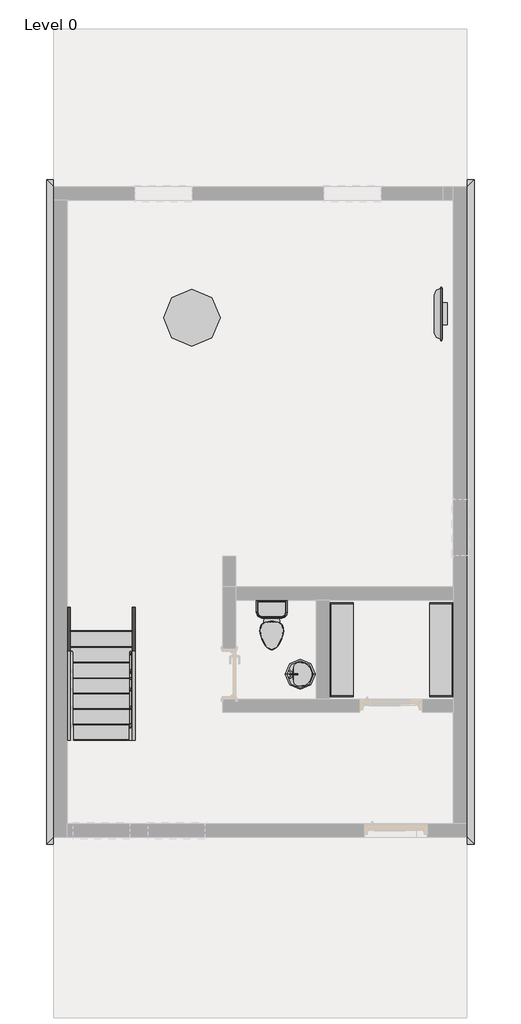
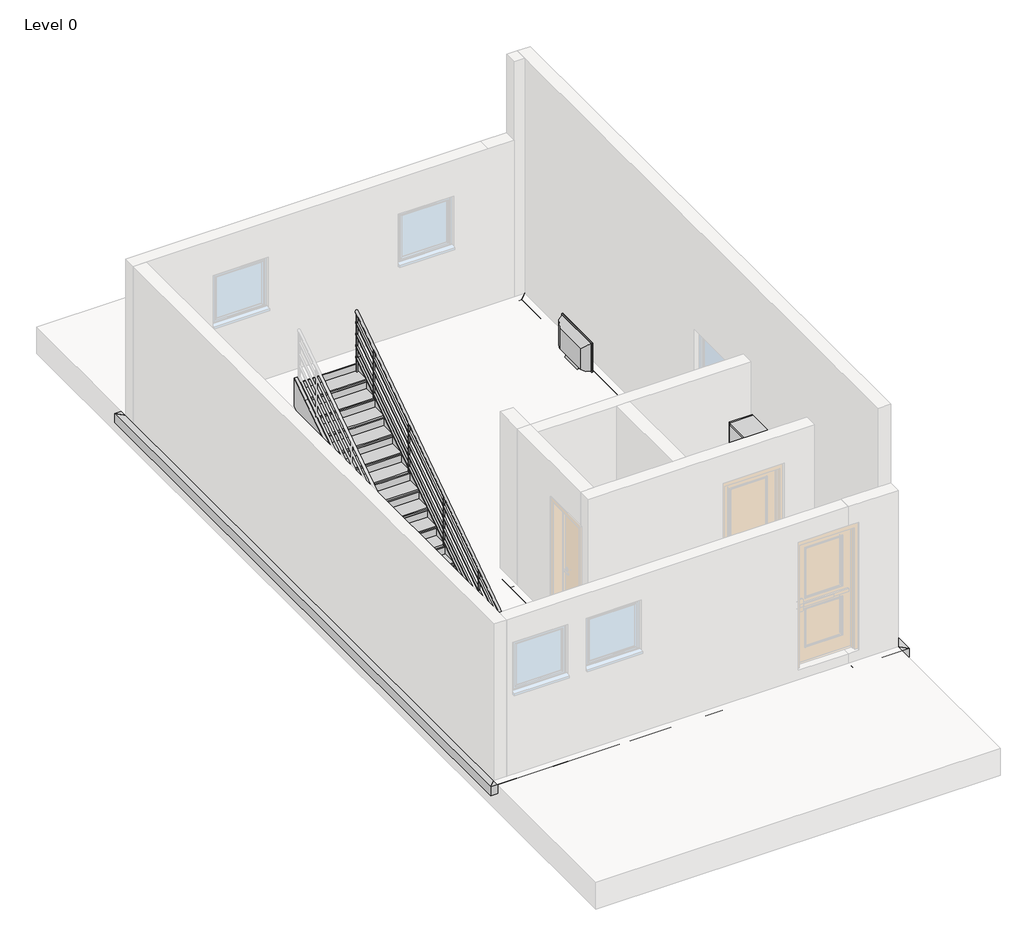
# One storey, part 2 of 2: 13 proxies, 2 flow terminals, 2 furniture elements, 2 members, 1 railing, 1 stair flight.
"""IFC4 building model written with IfcOpenShell, lengths in millimetres."""

from ifc_helpers import new_model, si_unit, frame, origin, place, context, project, spatial, polyline, circle_curve, ellipse_curve, outline, extrude, faceted_brep, transform, mapped, element, save
from ifc_brep_helpers import plane_surface, cylinder_surface, advanced_brep
from components import proxy_420707f7, flow_terminal_a43f4bde, toilet_domestic_3d_toilet_domestic_3d_ba6479b0, toilet_domestic_3d_toilet_domestic_3d_30431060, furniture_51289c3c, furniture_ec754799, wood_steps_w_50mm_tread_10mm_nosing_13mm_riser_22d6e456

model = new_model("IFC4")

# Units and contexts
model_context = context("Model", 3, world=origin())
ifc_project = project(units=[si_unit("LENGTHUNIT", "METRE", prefix="MILLI")], contexts=[model_context])

# Site, building, storey
site = spatial("IfcSite", under=ifc_project)
building = spatial("IfcBuilding", under=site)
storey = spatial("IfcBuildingStorey", under=building, Name="Level 0", Elevation=0.0)

# Proxies
placement = place(None, origin())
element("IfcBuildingElementProxy", 1, Name="Wall Sweeps", at=placement, inside=storey, context=model_context, shape_type="Brep", body=[
    faceted_brep([(-7042.7000057, 19249.9990528, 0.0), (-7042.7000057, 19249.9990528, -150.0), (-6592.7000057, 18799.9990528, -150.0), (-6592.7000057, 18799.9990528, 0.0), (-644.8785855, 19249.9990528, 0.0), (-644.8785855, 19132.4990528, 0.0), (-644.8785855, 18917.4990528, 0.0), (-644.8785855, 18799.9990528, 0.0), (-644.8785855, 18799.9990528, -150.0), (-644.8785855, 19249.9990528, -150.0)], [[[0, 1, 2, 3]], [[4, 5, 6, 7, 8, 9]], [[1, 0, 4, 9]], [[2, 1, 9, 8]], [[3, 2, 8, 7]], [[0, 3, 7, 6, 5, 4]]]),
])
element("IfcBuildingElementProxy", 2, Name="Wall Sweeps", at=placement, inside=storey, context=model_context, shape_type="SweptSolid", body=[
    extrude(outline(polyline([(-6592.7000057, 8959.9990528), (-7042.7000057, 8509.9990528), (-7042.7000057, 19249.9990528), (-6592.7000057, 18799.9990528), (-6592.7000057, 8959.9990528)])), frame((0.0, 0.0, -150.0), z_axis=(0.0, 0.0, 1.0), x_axis=(1.0, 0.0, 0.0)), (0.0, 0.0, 1.0), 150.0),
])
element("IfcBuildingElementProxy", 3, Name="Wall Sweeps", at=placement, inside=storey, context=model_context, shape_type="Brep", body=[
    faceted_brep([(-137.7000057, 8509.9990528, 0.0), (-137.7000057, 8509.9990528, -150.0), (-587.7000057, 8959.9990528, -150.0), (-587.7000057, 8959.9990528, 0.0), (-1075.2000057, 8509.9990528, 0.0), (-1075.2000057, 8627.4990528, 0.0), (-1075.2000057, 8842.4990528, 0.0), (-1075.2000057, 8959.9990528, 0.0), (-1075.2000057, 8959.9990528, -150.0), (-1075.2000057, 8509.9990528, -150.0)], [[[0, 1, 2, 3]], [[4, 5, 6, 7, 8, 9]], [[1, 0, 4, 9]], [[2, 1, 9, 8]], [[3, 2, 8, 7]], [[0, 3, 7, 6, 5, 4]]]),
])
element("IfcBuildingElementProxy", 4, Name="Wall Sweeps", at=placement, inside=storey, context=model_context, shape_type="SweptSolid", body=[
    extrude(outline(polyline([(-587.7000057, 18799.9990528), (-137.7000057, 19249.9990528), (-137.7000057, 8509.9990528), (-587.7000057, 8959.9990528), (-587.7000057, 18799.9990528)])), frame((0.0, 0.0, -150.0), z_axis=(0.0, 0.0, 1.0), x_axis=(1.0, 0.0, 0.0)), (0.0, 0.0, 1.0), 150.0),
])
element("IfcBuildingElementProxy", 5, Name="Wall Sweeps", at=placement, inside=storey, context=model_context, shape_type="Brep", body=[
    faceted_brep([(-1987.7250057, 10524.9990528, 0.0), (-1987.7250057, 10524.9990528, -150.0), (-1987.7250057, 10974.9990528, -150.0), (-1987.7250057, 10974.9990528, 0.0), (-1987.7250057, 10857.4990528, 0.0), (-1987.7250057, 10642.4990528, 0.0), (-4200.2000057, 10524.9990528, 0.0), (-4200.2000057, 10642.4990528, 0.0), (-4200.2000057, 10857.4990528, 0.0), (-4200.2000057, 10974.9990528, 0.0), (-4200.2000057, 10974.9990528, -150.0), (-4200.2000057, 10524.9990528, -150.0)], [[[0, 1, 2, 3, 4, 5]], [[6, 7, 8, 9, 10, 11]], [[1, 0, 6, 11]], [[2, 1, 11, 10]], [[3, 2, 10, 9]], [[0, 5, 4, 3, 9, 8, 7, 6]]]),
    faceted_brep([(-470.2000057, 10524.9990528, 0.0), (-470.2000057, 10524.9990528, -150.0), (-470.2000057, 10974.9990528, -150.0), (-470.2000057, 10974.9990528, 0.0), (-470.2000057, 10857.4990528, 0.0), (-470.2000057, 10642.4990528, 0.0), (-971.7250057, 10524.9990528, 0.0), (-971.7250057, 10642.4990528, 0.0), (-971.7250057, 10857.4990528, 0.0), (-971.7250057, 10974.9990528, 0.0), (-971.7250057, 10974.9990528, -150.0), (-971.7250057, 10524.9990528, -150.0)], [[[0, 1, 2, 3, 4, 5]], [[6, 7, 8, 9, 10, 11]], [[1, 0, 6, 11]], [[2, 1, 11, 10]], [[3, 2, 10, 9]], [[0, 5, 4, 3, 9, 8, 7, 6]]]),
])
element("IfcBuildingElementProxy", 6, Name="Wall Sweeps", at=placement, inside=storey, context=model_context, shape_type="Brep", body=[
    faceted_brep([(-4317.7000057, 11667.4990528, 0.0), (-4317.7000057, 11667.4990528, -150.0), (-3867.7000057, 11667.4990528, -150.0), (-3867.7000057, 11667.4990528, 0.0), (-3985.2000057, 11667.4990528, 0.0), (-4200.2000057, 11667.4990528, 0.0), (-4317.7000057, 12672.4990528, 0.0), (-4200.2000057, 12672.4990528, 0.0), (-3985.2000057, 12672.4990528, 0.0), (-3867.7000057, 12672.4990528, 0.0), (-3867.7000057, 12672.4990528, -150.0), (-4317.7000057, 12672.4990528, -150.0)], [[[0, 1, 2, 3, 4, 5]], [[6, 7, 8, 9, 10, 11]], [[1, 0, 6, 11]], [[2, 1, 11, 10]], [[3, 2, 10, 9]], [[0, 5, 4, 3, 9, 8, 7, 6]]]),
])
element("IfcBuildingElementProxy", 7, Name="Wall Sweeps", at=placement, inside=storey, context=model_context, shape_type="Brep", body=[
    faceted_brep([(-3985.2000057, 12339.9990528, 0.0), (-3985.2000057, 12457.4990528, 0.0), (-3985.2000057, 12672.4990528, 0.0), (-3985.2000057, 12789.9990528, 0.0), (-3985.2000057, 12789.9990528, -150.0), (-3985.2000057, 12339.9990528, -150.0), (-470.2000057, 12339.9990528, 0.0), (-470.2000057, 12339.9990528, -150.0), (-470.2000057, 12789.9990528, -150.0), (-470.2000057, 12789.9990528, 0.0), (-470.2000057, 12672.4990528, 0.0), (-470.2000057, 12457.4990528, 0.0)], [[[0, 1, 2, 3, 4, 5]], [[6, 7, 8, 9, 10, 11]], [[3, 2, 1, 0, 6, 11, 10, 9]], [[4, 3, 9, 8]], [[5, 4, 8, 7]], [[0, 5, 7, 6]]]),
])
element("IfcBuildingElementProxy", 8, Name="Wall Sweeps", at=placement, inside=storey, context=model_context, shape_type="Brep", body=[
    faceted_brep([(-2352.7000057, 12457.4990528, 0.0), (-2352.7000057, 12457.4990528, -150.0), (-2802.7000057, 12457.4990528, -150.0), (-2802.7000057, 12457.4990528, 0.0), (-2685.2000057, 12457.4990528, 0.0), (-2470.2000057, 12457.4990528, 0.0), (-2352.7000057, 10857.4990528, 0.0), (-2470.2000057, 10857.4990528, 0.0), (-2685.2000057, 10857.4990528, 0.0), (-2802.7000057, 10857.4990528, 0.0), (-2802.7000057, 10857.4990528, -150.0), (-2352.7000057, 10857.4990528, -150.0)], [[[0, 1, 2, 3, 4, 5]], [[6, 7, 8, 9, 10, 11]], [[1, 0, 6, 11]], [[2, 1, 11, 10]], [[3, 2, 10, 9]], [[0, 5, 4, 3, 9, 8, 7, 6]]]),
])
element("IfcBuildingElementProxy", 9, Name="Wall Sweeps", at=placement, inside=storey, context=model_context, shape_type="Brep", body=[
    faceted_brep([(-4317.7000057, 12672.4990528, 0.0), (-4317.7000057, 12672.4990528, -150.0), (-3867.7000057, 12672.4990528, -150.0), (-3867.7000057, 12672.4990528, 0.0), (-3985.2000057, 12672.4990528, 0.0), (-4200.2000057, 12672.4990528, 0.0), (-4317.7000057, 13164.9990528, 0.0), (-4200.2000057, 13164.9990528, 0.0), (-3985.2000057, 13164.9990528, 0.0), (-3867.7000057, 13164.9990528, 0.0), (-3867.7000057, 13164.9990528, -150.0), (-4317.7000057, 13164.9990528, -150.0)], [[[0, 1, 2, 3, 4, 5]], [[6, 7, 8, 9, 10, 11]], [[1, 0, 6, 11]], [[2, 1, 11, 10]], [[3, 2, 10, 9]], [[0, 5, 4, 3, 9, 8, 7, 6]]]),
])
element("IfcBuildingElementProxy", 10, Name="Wall Sweeps", at=placement, inside=storey, context=model_context, shape_type="Brep", body=[
    faceted_brep([(-1075.2000057, 8509.9990528, 0.0), (-1075.2000057, 8509.9990528, -150.0), (-1075.2000057, 8959.9990528, -150.0), (-1075.2000057, 8959.9990528, 0.0), (-1075.2000057, 8842.4990528, 0.0), (-1075.2000057, 8627.4990528, 0.0), (-7042.7000057, 8509.9990528, 0.0), (-6592.7000057, 8959.9990528, 0.0), (-6592.7000057, 8959.9990528, -150.0), (-7042.7000057, 8509.9990528, -150.0)], [[[0, 1, 2, 3, 4, 5]], [[6, 7, 8, 9]], [[1, 0, 6, 9]], [[2, 1, 9, 8]], [[3, 2, 8, 7]], [[0, 5, 4, 3, 7, 6]]]),
])
element("IfcBuildingElementProxy", 11, Name="Wall Sweeps", at=placement, inside=storey, context=model_context, shape_type="Brep", body=[
    faceted_brep([(-644.8785855, 19249.9990528, 0.0), (-644.8785855, 19249.9990528, -150.0), (-644.8785855, 18799.9990528, -150.0), (-644.8785855, 18799.9990528, 0.0), (-644.8785855, 18917.4990528, 0.0), (-644.8785855, 19132.4990528, 0.0), (-137.7000057, 19249.9990528, 0.0), (-587.7000057, 18799.9990528, 0.0), (-587.7000057, 18799.9990528, -150.0), (-137.7000057, 19249.9990528, -150.0)], [[[0, 1, 2, 3, 4, 5]], [[6, 7, 8, 9]], [[1, 0, 6, 9]], [[2, 1, 9, 8]], [[3, 2, 8, 7]], [[0, 5, 4, 3, 7, 6]]]),
])
proxy_shape = proxy_420707f7(model_context)
element("IfcBuildingElementProxy", 12, Name="Shelf - Book : 15\" x 72\"", ObjectType="Shelf - Book : 15\" x 72\"", at=placement, inside=storey, context=model_context, shape_type="MappedRepresentation", body=[
    mapped(proxy_shape, transform((-2470.2000057, 10893.4990528, 0.0), x_axis=(0.0, 1.0, 0.0), y_axis=(-1.0, 0.0, 0.0), z_axis=(0.0, 0.0, 1.0))),
])
element("IfcBuildingElementProxy", 13, Name="Shelf - Book : 15\" x 72\"", ObjectType="Shelf - Book : 15\" x 72\"", at=placement, inside=storey, context=model_context, shape_type="MappedRepresentation", body=[
    mapped(proxy_shape, transform((-470.2000057, 12417.4990528, 0.0), x_axis=(0.0, -1.0, 0.0), y_axis=(1.0, 0.0, 0.0), z_axis=(0.0, 0.0, 1.0))),
])

# Flow terminals
flow_terminal_shape = flow_terminal_a43f4bde(model_context)
element("IfcFlowTerminal", 14, ObjectType="Sink Vanity-Round : 19\" x 19\"", at=placement, inside=storey, context=model_context, shape_type="MappedRepresentation", body=[
    mapped(flow_terminal_shape, transform((-2859.6463882, 11160.8473122, 0.0), x_axis=(0.0, 1.0, 0.0), y_axis=(-1.0, 0.0, 0.0), z_axis=(0.0, 0.0, 1.0))),
])
toilet_domestic_3d_toilet_domestic_3d_shape = toilet_domestic_3d_toilet_domestic_3d_ba6479b0(model_context)
toilet_domestic_3d_toilet_domestic_3d_2_shape = toilet_domestic_3d_toilet_domestic_3d_30431060(model_context)
element("IfcFlowTerminal", 15, ObjectType="Toilet-Domestic-3D : Toilet-Domestic-3D", at=placement, inside=storey, context=model_context, shape_type="MappedRepresentation", body=[
    mapped(toilet_domestic_3d_toilet_domestic_3d_shape, transform((-3405.2000057, 11962.8030254, 0.0), x_axis=(1.0, 0.0, 0.0), y_axis=(0.0, 1.0, 0.0), z_axis=(0.0, 0.0, 1.0))),
    mapped(toilet_domestic_3d_toilet_domestic_3d_2_shape, transform((-3405.2000057, 11962.8030254, 0.0), x_axis=(1.0, 0.0, 0.0), y_axis=(0.0, 1.0, 0.0), z_axis=(0.0, 0.0, 1.0))),
])

# Furniture
furniture_shape = furniture_51289c3c(model_context)
element("IfcFurniture", 16, ObjectType="TV - Flat Screen : 32\"", at=placement, inside=storey, context=model_context, shape_type="MappedRepresentation", body=[
    mapped(furniture_shape, transform((-724.0620619, 17083.2435669, 0.0), x_axis=(0.0, 1.0, 0.0), y_axis=(-1.0, 0.0, 0.0), z_axis=(0.0, 0.0, 1.0))),
])
furniture_2_shape = furniture_ec754799(model_context)
element("IfcFurniture", 17, ObjectType="Table-Dining Round : 36\" Diameter", at=placement, inside=storey, context=model_context, shape_type="MappedRepresentation", body=[
    mapped(furniture_2_shape, transform((-4799.1819729, 17202.3777413, 0.0), x_axis=(1.0, 0.0, 0.0), y_axis=(0.0, 1.0, 0.0), z_axis=(0.0, 0.0, 1.0))),
])

# Members
element("IfcMember", 18, ObjectType="Stringer-50mm_Width", at=placement, inside=storey, context=model_context, shape_type="SweptSolid", body=[
    extrude(outline(polyline([(10192.4990528, 0.0), (10192.4990528, 233.8698899), (14692.4990528, 3265.4488372), (14692.4990528, 2783.1459589), (10561.2667701, 0.0), (10192.4990528, 0.0)])), frame((-6710.2000057, 0.0, 0.0), z_axis=(1.0, 0.0, 0.0), x_axis=(0.0, 1.0, 0.0)), (0.0, 0.0, 1.0), 50.0),
])
element("IfcMember", 19, ObjectType="Stringer-50mm_Width", at=placement, inside=storey, context=model_context, shape_type="SweptSolid", body=[
    extrude(outline(polyline([(10192.4990528, 0.0), (10192.4990528, 233.8698899), (14692.4990528, 3265.4488372), (14692.4990528, 2783.1459589), (10561.2667701, 0.0), (10192.4990528, 0.0)])), frame((-5660.2000057, 0.0, 0.0), z_axis=(1.0, 0.0, 0.0), x_axis=(0.0, 1.0, 0.0)), (0.0, 0.0, 1.0), 50.0),
])

# Railing
element("IfcRailing", 20, ObjectType="900mm_Pipe", at=placement, inside=storey, context=model_context, shape_type="AdvancedBrep", body=[
    advanced_brep(
    [(-5665.6000057, 10192.4990528, 1044.3059087), (-5705.6000057, 10192.4990528, 1044.3059087), (-5665.6000057, 14692.4990528, 4075.8848561), (-5705.6000057, 14692.4990528, 4075.8848561)],
    [
        (0, 1, ellipse_curve(frame((-5685.6000057, 10192.4990528, 1044.3059087), z_axis=(0.0, -1.0, 0.0), x_axis=(0.0, 0.0, -1.0)), 24.1151439, 20.0)),
        (1, 0, ellipse_curve(frame((-5685.6000057, 10192.4990528, 1044.3059087), z_axis=(0.0, -1.0, 0.0), x_axis=(0.0, 0.0, -1.0)), 24.1151439, 20.0)),
        (2, 3, ellipse_curve(frame((-5685.6000057, 14692.4990528, 4075.8848561), z_axis=(0.0, 1.0, 0.0), x_axis=(0.0, 0.0, -1.0)), 24.1151439, 20.0)),
        (3, 2, ellipse_curve(frame((-5685.6000057, 14692.4990528, 4075.8848561), z_axis=(0.0, 1.0, 0.0), x_axis=(0.0, 0.0, -1.0)), 24.1151439, 20.0)),
        (0, 2),
        (3, 1),
    ],
    [
        plane_surface(frame((-5685.6000057, 10192.4990528, 1068.4210526), z_axis=(0.0, -1.0, 0.0), x_axis=(0.0, 0.0, 1.0))),
        plane_surface(frame((-5685.6000057, 14692.4990528, 4100.0), z_axis=(0.0, 1.0, 0.0), x_axis=(0.0, 0.0, 1.0))),
        cylinder_surface(frame((-5685.6000057, 10203.6735117, 1051.8339652), z_axis=(0.0, -0.8293543703358371, -0.5587229442262482), x_axis=(-1.0, 0.0, 0.0)), 20.0),
    ],
    [
        (0, [[1, 2]]),
        (1, [[3, 4]]),
        (2, [[-1, 5, -4, 6]]),
        (2, [[-2, -6, -3, -5]]),
    ],
),
    advanced_brep(
    [(-5700.6000057, 10192.4990528, 850.3346947), (-5670.6000057, 10192.4990528, 850.3346947), (-5700.6000057, 14692.4990528, 3881.9136421), (-5670.6000057, 14692.4990528, 3881.9136421)],
    [
        (0, 1, ellipse_curve(frame((-5685.6000057, 10192.4990528, 850.3346947), z_axis=(0.0, -1.0, 0.0), x_axis=(0.0, 0.0, -1.0)), 18.0863579, 15.0)),
        (1, 0, ellipse_curve(frame((-5685.6000057, 10192.4990528, 850.3346947), z_axis=(0.0, -1.0, 0.0), x_axis=(0.0, 0.0, -1.0)), 18.0863579, 15.0)),
        (2, 3, ellipse_curve(frame((-5685.6000057, 14692.4990528, 3881.9136421), z_axis=(0.0, 1.0, 0.0), x_axis=(0.0, 0.0, -1.0)), 18.0863579, 15.0)),
        (3, 2, ellipse_curve(frame((-5685.6000057, 14692.4990528, 3881.9136421), z_axis=(0.0, 1.0, 0.0), x_axis=(0.0, 0.0, -1.0)), 18.0863579, 15.0)),
        (0, 2),
        (3, 1),
    ],
    [
        plane_surface(frame((-5685.6000057, 10192.4990528, 868.4210526), z_axis=(0.0, -1.0, 0.0), x_axis=(0.0, 0.0, 1.0))),
        plane_surface(frame((-5685.6000057, 14692.4990528, 3900.0), z_axis=(0.0, 1.0, 0.0), x_axis=(0.0, 0.0, 1.0))),
        cylinder_surface(frame((-5685.6000057, 10200.879897, 855.9807371), z_axis=(0.0, -0.8293543703358371, -0.5587229442262482), x_axis=(1.0, 0.0, 0.0)), 15.0),
    ],
    [
        (0, [[1, 2]]),
        (1, [[3, 4]]),
        (2, [[-1, 5, -4, 6]]),
        (2, [[-2, -6, -3, -5]]),
    ],
),
    advanced_brep(
    [(-5700.6000057, 10192.4990528, 650.3346947), (-5670.6000057, 10192.4990528, 650.3346947), (-5700.6000057, 14692.4990528, 3681.9136421), (-5670.6000057, 14692.4990528, 3681.9136421)],
    [
        (0, 1, ellipse_curve(frame((-5685.6000057, 10192.4990528, 650.3346947), z_axis=(0.0, -1.0, 0.0), x_axis=(0.0, 0.0, -1.0)), 18.0863579, 15.0)),
        (1, 0, ellipse_curve(frame((-5685.6000057, 10192.4990528, 650.3346947), z_axis=(0.0, -1.0, 0.0), x_axis=(0.0, 0.0, -1.0)), 18.0863579, 15.0)),
        (2, 3, ellipse_curve(frame((-5685.6000057, 14692.4990528, 3681.9136421), z_axis=(0.0, 1.0, 0.0), x_axis=(0.0, 0.0, -1.0)), 18.0863579, 15.0)),
        (3, 2, ellipse_curve(frame((-5685.6000057, 14692.4990528, 3681.9136421), z_axis=(0.0, 1.0, 0.0), x_axis=(0.0, 0.0, -1.0)), 18.0863579, 15.0)),
        (0, 2),
        (3, 1),
    ],
    [
        plane_surface(frame((-5685.6000057, 10192.4990528, 668.4210526), z_axis=(0.0, -1.0, 0.0), x_axis=(0.0, 0.0, 1.0))),
        plane_surface(frame((-5685.6000057, 14692.4990528, 3700.0), z_axis=(0.0, 1.0, 0.0), x_axis=(0.0, 0.0, 1.0))),
        cylinder_surface(frame((-5685.6000057, 10200.879897, 655.9807371), z_axis=(0.0, -0.8293543703358371, -0.5587229442262482), x_axis=(1.0, 0.0, 0.0)), 15.0),
    ],
    [
        (0, [[1, 2]]),
        (1, [[3, 4]]),
        (2, [[-1, 5, -4, 6]]),
        (2, [[-2, -6, -3, -5]]),
    ],
),
    advanced_brep(
    [(-5700.6000057, 10192.4990528, 450.3346947), (-5670.6000057, 10192.4990528, 450.3346947), (-5700.6000057, 14692.4990528, 3481.9136421), (-5670.6000057, 14692.4990528, 3481.9136421)],
    [
        (0, 1, ellipse_curve(frame((-5685.6000057, 10192.4990528, 450.3346947), z_axis=(0.0, -1.0, 0.0), x_axis=(0.0, 0.0, -1.0)), 18.0863579, 15.0)),
        (1, 0, ellipse_curve(frame((-5685.6000057, 10192.4990528, 450.3346947), z_axis=(0.0, -1.0, 0.0), x_axis=(0.0, 0.0, -1.0)), 18.0863579, 15.0)),
        (2, 3, ellipse_curve(frame((-5685.6000057, 14692.4990528, 3481.9136421), z_axis=(0.0, 1.0, 0.0), x_axis=(0.0, 0.0, -1.0)), 18.0863579, 15.0)),
        (3, 2, ellipse_curve(frame((-5685.6000057, 14692.4990528, 3481.9136421), z_axis=(0.0, 1.0, 0.0), x_axis=(0.0, 0.0, -1.0)), 18.0863579, 15.0)),
        (0, 2),
        (3, 1),
    ],
    [
        plane_surface(frame((-5685.6000057, 10192.4990528, 468.4210526), z_axis=(0.0, -1.0, 0.0), x_axis=(0.0, 0.0, 1.0))),
        plane_surface(frame((-5685.6000057, 14692.4990528, 3500.0), z_axis=(0.0, 1.0, 0.0), x_axis=(0.0, 0.0, 1.0))),
        cylinder_surface(frame((-5685.6000057, 10200.879897, 455.9807371), z_axis=(0.0, -0.8293543703358371, -0.5587229442262482), x_axis=(1.0, 0.0, 0.0)), 15.0),
    ],
    [
        (0, [[1, 2]]),
        (1, [[3, 4]]),
        (2, [[-1, 5, -4, 6]]),
        (2, [[-2, -6, -3, -5]]),
    ],
),
    advanced_brep(
    [(-5700.6000057, 10192.4990528, 250.3346947), (-5670.6000057, 10192.4990528, 250.3346947), (-5700.6000057, 14692.4990528, 3281.9136421), (-5670.6000057, 14692.4990528, 3281.9136421)],
    [
        (0, 1, ellipse_curve(frame((-5685.6000057, 10192.4990528, 250.3346947), z_axis=(0.0, -1.0, 0.0), x_axis=(0.0, 0.0, -1.0)), 18.0863579, 15.0)),
        (1, 0, ellipse_curve(frame((-5685.6000057, 10192.4990528, 250.3346947), z_axis=(0.0, -1.0, 0.0), x_axis=(0.0, 0.0, -1.0)), 18.0863579, 15.0)),
        (2, 3, ellipse_curve(frame((-5685.6000057, 14692.4990528, 3281.9136421), z_axis=(0.0, 1.0, 0.0), x_axis=(0.0, 0.0, -1.0)), 18.0863579, 15.0)),
        (3, 2, ellipse_curve(frame((-5685.6000057, 14692.4990528, 3281.9136421), z_axis=(0.0, 1.0, 0.0), x_axis=(0.0, 0.0, -1.0)), 18.0863579, 15.0)),
        (0, 2),
        (3, 1),
    ],
    [
        plane_surface(frame((-5685.6000057, 10192.4990528, 268.4210526), z_axis=(0.0, -1.0, 0.0), x_axis=(0.0, 0.0, 1.0))),
        plane_surface(frame((-5685.6000057, 14692.4990528, 3300.0), z_axis=(0.0, 1.0, 0.0), x_axis=(0.0, 0.0, 1.0))),
        cylinder_surface(frame((-5685.6000057, 10200.879897, 255.9807371), z_axis=(0.0, -0.8293543703358371, -0.5587229442262482), x_axis=(1.0, 0.0, 0.0)), 15.0),
    ],
    [
        (0, [[1, 2]]),
        (1, [[3, 4]]),
        (2, [[-1, 5, -4, 6]]),
        (2, [[-2, -6, -3, -5]]),
    ],
),
    advanced_brep(
    [(-5673.1000057, 14192.4990528, 3714.9276069), (-5673.1000057, 14192.4990528, 2863.1578947), (-5698.1000057, 14192.4990528, 2863.1578947), (-5698.1000057, 14192.4990528, 3714.9276069)],
    [
        (0, 1),
        (1, 2, circle_curve(frame((-5685.6000057, 14192.4990528, 2863.1578947), z_axis=(0.0, 0.0, 1.0), x_axis=(-1.0, 0.0, 0.0)), 12.5)),
        (2, 3),
        (3, 0, ellipse_curve(frame((-5685.6000057, 14192.4990528, 3714.9276069), z_axis=(0.0, 0.5587229442262482, -0.829354370335837), x_axis=(0.0, 0.8293543703358369, 0.5587229442262482)), 15.0719649, 12.5)),
        (0, 3, ellipse_curve(frame((-5685.6000057, 14192.4990528, 3714.9276069), z_axis=(0.0, 0.5587229442262482, -0.829354370335837), x_axis=(0.0, 0.8293543703358369, 0.5587229442262482)), 15.0719649, 12.5)),
        (2, 1, circle_curve(frame((-5685.6000057, 14192.4990528, 2863.1578947), z_axis=(0.0, 0.0, 1.0), x_axis=(-1.0, 0.0, 0.0)), 12.5)),
    ],
    [
        cylinder_surface(frame((-5685.6000057, 14192.4990528, 2763.1578947), z_axis=(0.0, 0.0, 1.0), x_axis=(-1.0, 0.0, 0.0)), 12.5),
        plane_surface(frame((-5710.6000057, 14217.4990528, 3731.7697122), z_axis=(0.0, -0.5587229442262482, 0.829354370335837), x_axis=(1.0, 0.0, 0.0))),
        plane_surface(frame((-5710.6000057, 14167.4990528, 2863.1578947), z_axis=(0.0, 0.0, -1.0), x_axis=(1.0, 0.0, 0.0))),
    ],
    [
        (0, [[1, 2, 3, 4]]),
        (0, [[-1, 5, -3, 6]]),
        (1, [[-4, -5]]),
        (2, [[-2, -6]]),
    ],
),
    advanced_brep(
    [(-5673.1000057, 13192.4990528, 3041.2433964), (-5673.1000057, 13192.4990528, 2189.4736842), (-5698.1000057, 13192.4990528, 2189.4736842), (-5698.1000057, 13192.4990528, 3041.2433964)],
    [
        (0, 1),
        (1, 2, circle_curve(frame((-5685.6000057, 13192.4990528, 2189.4736842), z_axis=(0.0, 0.0, 1.0), x_axis=(-1.0, 0.0, 0.0)), 12.5)),
        (2, 3),
        (3, 0, ellipse_curve(frame((-5685.6000057, 13192.4990528, 3041.2433964), z_axis=(0.0, 0.5587229442262482, -0.829354370335837), x_axis=(0.0, 0.8293543703358369, 0.5587229442262482)), 15.0719649, 12.5)),
        (0, 3, ellipse_curve(frame((-5685.6000057, 13192.4990528, 3041.2433964), z_axis=(0.0, 0.5587229442262482, -0.829354370335837), x_axis=(0.0, 0.8293543703358369, 0.5587229442262482)), 15.0719649, 12.5)),
        (2, 1, circle_curve(frame((-5685.6000057, 13192.4990528, 2189.4736842), z_axis=(0.0, 0.0, 1.0), x_axis=(-1.0, 0.0, 0.0)), 12.5)),
    ],
    [
        cylinder_surface(frame((-5685.6000057, 13192.4990528, 2089.4736842), z_axis=(0.0, 0.0, 1.0), x_axis=(-1.0, 0.0, 0.0)), 12.5),
        plane_surface(frame((-5710.6000057, 13217.4990528, 3058.0855016), z_axis=(0.0, -0.5587229442262482, 0.829354370335837), x_axis=(1.0, 0.0, 0.0))),
        plane_surface(frame((-5710.6000057, 13167.4990528, 2189.4736842), z_axis=(0.0, 0.0, -1.0), x_axis=(1.0, 0.0, 0.0))),
    ],
    [
        (0, [[1, 2, 3, 4]]),
        (0, [[-1, 5, -3, 6]]),
        (1, [[-4, -5]]),
        (2, [[-2, -6]]),
    ],
),
    advanced_brep(
    [(-5673.1000057, 12192.4990528, 2367.5591858), (-5673.1000057, 12192.4990528, 1515.7894737), (-5698.1000057, 12192.4990528, 1515.7894737), (-5698.1000057, 12192.4990528, 2367.5591858)],
    [
        (0, 1),
        (1, 2, circle_curve(frame((-5685.6000057, 12192.4990528, 1515.7894737), z_axis=(0.0, 0.0, 1.0), x_axis=(-1.0, 0.0, 0.0)), 12.5)),
        (2, 3),
        (3, 0, ellipse_curve(frame((-5685.6000057, 12192.4990528, 2367.5591858), z_axis=(0.0, 0.5587229442262482, -0.829354370335837), x_axis=(0.0, 0.8293543703358369, 0.5587229442262482)), 15.0719649, 12.5)),
        (0, 3, ellipse_curve(frame((-5685.6000057, 12192.4990528, 2367.5591858), z_axis=(0.0, 0.5587229442262482, -0.829354370335837), x_axis=(0.0, 0.8293543703358369, 0.5587229442262482)), 15.0719649, 12.5)),
        (2, 1, circle_curve(frame((-5685.6000057, 12192.4990528, 1515.7894737), z_axis=(0.0, 0.0, 1.0), x_axis=(-1.0, 0.0, 0.0)), 12.5)),
    ],
    [
        cylinder_surface(frame((-5685.6000057, 12192.4990528, 1415.7894737), z_axis=(0.0, 0.0, 1.0), x_axis=(-1.0, 0.0, 0.0)), 12.5),
        plane_surface(frame((-5710.6000057, 12217.4990528, 2384.4012911), z_axis=(0.0, -0.5587229442262482, 0.829354370335837), x_axis=(1.0, 0.0, 0.0))),
        plane_surface(frame((-5710.6000057, 12167.4990528, 1515.7894737), z_axis=(0.0, 0.0, -1.0), x_axis=(1.0, 0.0, 0.0))),
    ],
    [
        (0, [[1, 2, 3, 4]]),
        (0, [[-1, 5, -3, 6]]),
        (1, [[-4, -5]]),
        (2, [[-2, -6]]),
    ],
),
    advanced_brep(
    [(-5673.1000057, 11192.4990528, 1693.8749753), (-5673.1000057, 11192.4990528, 842.1052632), (-5698.1000057, 11192.4990528, 842.1052632), (-5698.1000057, 11192.4990528, 1693.8749753)],
    [
        (0, 1),
        (1, 2, circle_curve(frame((-5685.6000057, 11192.4990528, 842.1052632), z_axis=(0.0, 0.0, 1.0), x_axis=(-1.0, 0.0, 0.0)), 12.5)),
        (2, 3),
        (3, 0, ellipse_curve(frame((-5685.6000057, 11192.4990528, 1693.8749753), z_axis=(0.0, 0.5587229442262482, -0.829354370335837), x_axis=(0.0, 0.8293543703358369, 0.5587229442262482)), 15.0719649, 12.5)),
        (0, 3, ellipse_curve(frame((-5685.6000057, 11192.4990528, 1693.8749753), z_axis=(0.0, 0.5587229442262482, -0.829354370335837), x_axis=(0.0, 0.8293543703358369, 0.5587229442262482)), 15.0719649, 12.5)),
        (2, 1, circle_curve(frame((-5685.6000057, 11192.4990528, 842.1052632), z_axis=(0.0, 0.0, 1.0), x_axis=(-1.0, 0.0, 0.0)), 12.5)),
    ],
    [
        cylinder_surface(frame((-5685.6000057, 11192.4990528, 742.1052632), z_axis=(0.0, 0.0, 1.0), x_axis=(-1.0, 0.0, 0.0)), 12.5),
        plane_surface(frame((-5710.6000057, 11217.4990528, 1710.7170806), z_axis=(0.0, -0.5587229442262482, 0.829354370335837), x_axis=(1.0, 0.0, 0.0))),
        plane_surface(frame((-5710.6000057, 11167.4990528, 842.1052632), z_axis=(0.0, 0.0, -1.0), x_axis=(1.0, 0.0, 0.0))),
    ],
    [
        (0, [[1, 2, 3, 4]]),
        (0, [[-1, 5, -3, 6]]),
        (1, [[-4, -5]]),
        (2, [[-2, -6]]),
    ],
),
    advanced_brep(
    [(-5673.1000057, 14679.9990528, 4043.3486595), (-5673.1000057, 14679.9990528, 3031.5789474), (-5698.1000057, 14679.9990528, 3031.5789474), (-5698.1000057, 14679.9990528, 4043.3486595)],
    [
        (0, 1),
        (1, 2, circle_curve(frame((-5685.6000057, 14679.9990528, 3031.5789474), z_axis=(0.0, 0.0, 1.0), x_axis=(-1.0, 0.0, 0.0)), 12.5)),
        (2, 3),
        (3, 0, ellipse_curve(frame((-5685.6000057, 14679.9990528, 4043.3486595), z_axis=(0.0, 0.5587229442262482, -0.829354370335837), x_axis=(0.0, 0.8293543703358369, 0.5587229442262482)), 15.0719649, 12.5)),
        (0, 3, ellipse_curve(frame((-5685.6000057, 14679.9990528, 4043.3486595), z_axis=(0.0, 0.5587229442262482, -0.829354370335837), x_axis=(0.0, 0.8293543703358369, 0.5587229442262482)), 15.0719649, 12.5)),
        (2, 1, circle_curve(frame((-5685.6000057, 14679.9990528, 3031.5789474), z_axis=(0.0, 0.0, 1.0), x_axis=(-1.0, 0.0, 0.0)), 12.5)),
    ],
    [
        cylinder_surface(frame((-5685.6000057, 14679.9990528, 2931.5789474), z_axis=(0.0, 0.0, 1.0), x_axis=(-1.0, 0.0, 0.0)), 12.5),
        plane_surface(frame((-5710.6000057, 14704.9990528, 4060.1907648), z_axis=(0.0, -0.5587229442262482, 0.829354370335837), x_axis=(1.0, 0.0, 0.0))),
        plane_surface(frame((-5710.6000057, 14654.9990528, 3031.5789474), z_axis=(0.0, 0.0, -1.0), x_axis=(1.0, 0.0, 0.0))),
    ],
    [
        (0, [[1, 2, 3, 4]]),
        (0, [[-1, 5, -3, 6]]),
        (1, [[-4, -5]]),
        (2, [[-2, -6]]),
    ],
),
    advanced_brep(
    [(-5673.1000057, 10204.9990528, 1028.6118174), (-5673.1000057, 10204.9990528, 168.4210526), (-5698.1000057, 10204.9990528, 168.4210526), (-5698.1000057, 10204.9990528, 1028.6118174)],
    [
        (0, 1),
        (1, 2, circle_curve(frame((-5685.6000057, 10204.9990528, 168.4210526), z_axis=(0.0, 0.0, 1.0), x_axis=(-1.0, 0.0, 0.0)), 12.5)),
        (2, 3),
        (3, 0, ellipse_curve(frame((-5685.6000057, 10204.9990528, 1028.6118174), z_axis=(0.0, 0.5587229442262482, -0.829354370335837), x_axis=(0.0, 0.8293543703358369, 0.5587229442262482)), 15.0719649, 12.5)),
        (0, 3, ellipse_curve(frame((-5685.6000057, 10204.9990528, 1028.6118174), z_axis=(0.0, 0.5587229442262482, -0.829354370335837), x_axis=(0.0, 0.8293543703358369, 0.5587229442262482)), 15.0719649, 12.5)),
        (2, 1, circle_curve(frame((-5685.6000057, 10204.9990528, 168.4210526), z_axis=(0.0, 0.0, 1.0), x_axis=(-1.0, 0.0, 0.0)), 12.5)),
    ],
    [
        cylinder_surface(frame((-5685.6000057, 10204.9990528, 68.4210526), z_axis=(0.0, 0.0, 1.0), x_axis=(-1.0, 0.0, 0.0)), 12.5),
        plane_surface(frame((-5710.6000057, 10229.9990528, 1045.4539227), z_axis=(0.0, -0.5587229442262482, 0.829354370335837), x_axis=(1.0, 0.0, 0.0))),
        plane_surface(frame((-5710.6000057, 10179.9990528, 168.4210526), z_axis=(0.0, 0.0, -1.0), x_axis=(1.0, 0.0, 0.0))),
    ],
    [
        (0, [[1, 2, 3, 4]]),
        (0, [[-1, 5, -3, 6]]),
        (1, [[-4, -5]]),
        (2, [[-2, -6]]),
    ],
),
])

# Stair flight
wood_steps_w_50mm_tread_10mm_nosing_13mm_riser_shape = wood_steps_w_50mm_tread_10mm_nosing_13mm_riser_22d6e456(model_context)
element("IfcStairFlight", 21, ObjectType="Wood_Steps_w-50mm_Tread-10mm_Nosing-13mm_Riser", at=placement, inside=storey, context=model_context, shape_type="MappedRepresentation", body=[
    mapped(wood_steps_w_50mm_tread_10mm_nosing_13mm_riser_shape, transform((0.0, 0.0, 0.0), x_axis=(1.0, 0.0, 0.0), y_axis=(0.0, 1.0, 0.0), z_axis=(0.0, 0.0, 1.0))),
])

save(model, "model.ifc")

# Revit data of these elements
# Type "Shelf - Book : 15\" x 72\""
#   Assembly Code = "E1010510"
#   Depth = 381 mm
#   Height = 1828.8 mm
#   Length [instance default] = 1524 mm
#   Base Material = Finishes - Paint - Black
#   Material = Laminate - Ivory,Matte
#   Default Elevation = 0
# Type "Sink Vanity-Round : 19\" x 19\""
#   Assembly Code = "D2010400"
#   Top Of Counter = 787.4 mm
#   Basin Material = Porcelain, Linen
#   Faucet Material = Steel, Polished
#   Default Elevation = 0
# Type "Toilet-Domestic-3D : Toilet-Domestic-3D"
#   Assembly Code = "D2010110"
#   Toilet - Bowl/Basin Material = Porcelain, Linen
#   Toilet - Seat Material = Laminate, Linen, Matte
#   Default Elevation = 0
# Type "TV - Flat Screen : 32\""
#   SinAng = 0.49 mm
#   L = 705.961 mm
#   H = 397.139 mm
#   Thickness = 110 mm
#   Diagonal = 810 mm
#   CosAng = 0.872 mm
#   Stand [instance default] = yes
#   Default Elevation = 0
# Type "Table-Dining Round : 36\" Diameter"
#   Assembly Code = "E2020200"
#   Diameter = 914.4 mm
#   Height = 762 mm
#   Base Material = Pine
#   Top Material = Laminate, Linen, Matte
#   Default Elevation = 0
# Type "900mm_Pipe"
#   built-in parameter 1008612 = 0.019685 (stored number, unit not read)
#   built-in parameter 1008611 = 0.0984252 (stored number, unit not read)
#   built-in parameter 1008609 = 3.28084 (stored number, unit not read)
#   built-in parameter 1008604 = 0.19685 (stored number, unit not read)
#   built-in parameter 1008603 = 0.164042 (stored number, unit not read)
#   Railing Height = 900 mm
#   built-in parameter 1008630 = 2
#   built-in parameter 1008610 = 1
#   built-in parameter 1008605 = 1
#   built-in parameter 1008618 = Baluster_Round : 25mm
# Elements 1, 2, 3, 4, 5, 6, 7, 8, 9, 10, 11 (IfcBuildingElementProxy)
#   Phase Created = New Construction
#   Materials on its faces: "Concrete, Cast In Situ"
# Elements 12, 13 (IfcBuildingElementProxy, "Shelf - Book : 15\" x 72\"")
#   Length = 1524 mm
#   Phase Created = New Construction
#   Materials on its faces: "Laminate - Ivory,Matte", "Finishes - Paint - Black"
# Element 14 (IfcFlowTerminal, "Sink Vanity-Round : 19\" x 19\"")
#   Mark = "2"
#   Phase Created = New Construction
#   Materials on its faces: "Porcelain, Linen", "Steel, Polished"
# Element 15 (IfcFlowTerminal, "Toilet-Domestic-3D : Toilet-Domestic-3D")
#   Mark = "1"
#   Phase Created = New Construction
#   Materials on its faces: "Porcelain, Linen", "Laminate, Linen, Matte"
# Element 16 (IfcFurniture, "TV - Flat Screen : 32\"")
#   Stand = yes
#   Phase Created = New Construction
#   Materials on its faces: "TV - Black", "TV - Glass", "TV - Screen"
# Element 17 (IfcFurniture, "Table-Dining Round : 36\" Diameter")
#   Phase Created = New Construction
#   Materials on its faces: "Pine", "Laminate, Linen, Matte"
# Elements 18, 19 (IfcMember, "Stringer-50mm_Width")
#   Phase Created = New Construction
# Element 20 (IfcRailing, "900mm_Pipe")
#   Phase Created = New Construction
# Element 21 (IfcStairFlight, "Wood_Steps_w-50mm_Tread-10mm_Nosing-13mm_Riser")
#   Phase Created = New Construction
#   Materials on its faces: "Oak Flooring"
# Materials
#   "Finishes - Paint - Black": colour RGB 0 0 0, transparency 0
#   "Laminate - Ivory,Matte": colour RGB 247 247 239, transparency 0
#   "Porcelain, Linen": class "Ceramic", colour RGB 249 239 230, transparency 0, Description = "Porcelain, linen", Cost = 0
#   "Steel, Polished": class "Metal", colour RGB 57 57 57, transparency 0, Description = "Polished steel", Cost = 0
#   "Laminate, Linen, Matte": class "Plastic", colour RGB 249 239 230, transparency 0, Description = "Plastic Laminate - Linen, Matte", Cost = 0
#   "Pine": class "Wood", colour RGB 223 192 134, transparency 0, Description = "Pinus Echinata", Cost = 0
#   "Concrete, Cast In Situ": class "Concrete", colour RGB 192 192 192, transparency 0, Description = "physical material", Cost = 0
#   "TV - Black": colour RGB 49 49 49, transparency 0
#   "TV - Glass": colour RGB 157 157 157, transparency 0.9
#   "TV - Screen": colour RGB 0 0 0, transparency 0
#   "Oak Flooring": class "Wood", colour RGB 212 179 113, transparency 0, Description = "Quercus Rubra", Cost = 0
